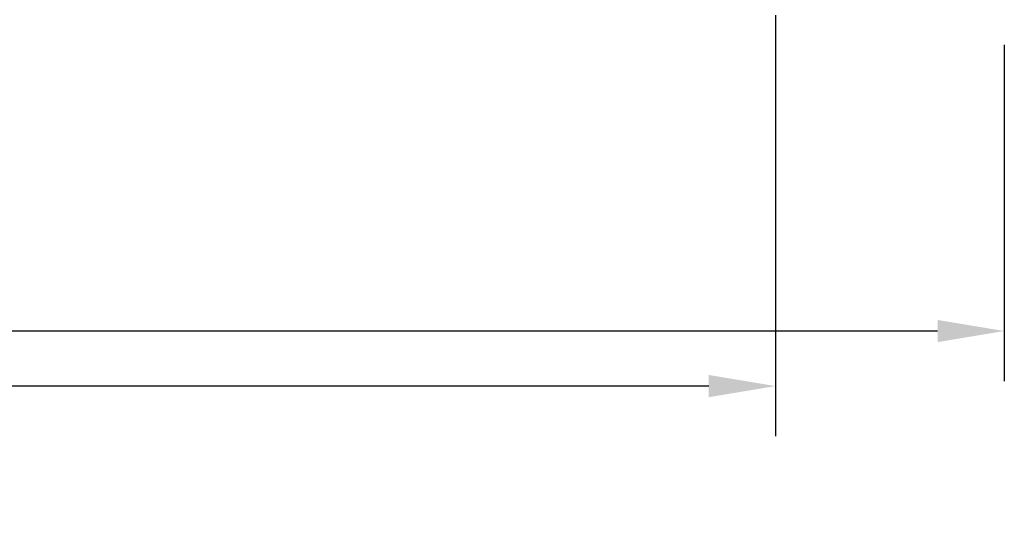
# Model space of a CAD drawing. Units: inches. Extents: x 89 to 490, y -59 to 378.
# Tile 13 of 20: x 400 to 459, y -59 to -28. Entities that reach past the tile are written whole.
import ezdxf

# ---------------------------------------------------------------- set-up
doc = ezdxf.new("R2010")
doc.units = ezdxf.units.IN
doc.header["$MEASUREMENT"] = 0
doc.layers.add('A-ANNO-DIMS', color=2, linetype='Continuous', lineweight=18)
doc.styles.get("Standard").update_dxf_attribs({"font": 'arial.ttf'})
doc.dimstyles.get("Standard").update_dxf_attribs({"dimtxt": 6, "dimasz": 4, "dimexe": 3, "dimexo": 3, "dimgap": 0.09, "dimtad": 0, "dimtih": 1, "dimtoh": 1, "dimdec": 1, "dimzin": 0, "dimdsep": 46, "dimlunit": 3, "dimtxsty": 'Standard', "dimcen": 0.09, "dimadec": 0, "dimazin": 0, "dimtfac": 1, "dimtdec": 1, "dimtofl": 0, "dimtmove": 0, "dimatfit": 3, "dimfxl": 1, "dimtolj": 1, "dimtzin": 0, "dimarcsym": 0})

# ---------------------------------------------------------------- blocks, each defined once
blk = doc.blocks.new('*D46')
at = {"layer": 'A-ANNO-DIMS', "color": 0, "lineweight": -2, "transparency": 16777216}
for p, q in [((277.443, -27.866), (277.443, -53.11)), ((445.739, -27.866), (445.739, -53.11)), ((281.443, -50.11), (332.892, -50.11)), ((441.739, -50.11), (390.289, -50.11))]:
    blk.add_line(p, q, dxfattribs=at)
at = {"layer": 'A-ANNO-DIMS', "color": 0, "transparency": 16777216}
for points in [[(281.443, -49.443), (281.443, -50.777), (277.443, -50.11)], [(441.739, -49.443), (441.739, -50.777), (445.739, -50.11)]]:
    blk.add_solid(points, dxfattribs=at)
at = {"layer": 'Defpoints', "color": 0, "transparency": 16777216}
for p in [(277.443, -24.866), (445.739, -24.866), (445.739, -50.11)]:
    blk.add_point(p, dxfattribs=at)
at = {"layer": 'A-ANNO-DIMS', "color": 0, "transparency": 16777216, "insert": (361.591, -50.11), "char_height": 6, "attachment_point": 5}
blk.add_mtext('\\A1;PLANTING 168', dxfattribs=at)
blk = doc.blocks.new('*D48')
at = {"layer": 'A-ANNO-DIMS', "color": 0, "lineweight": -2, "transparency": 16777216}
for p, q in [((127.441, 10.741), (127.441, -49.809)), ((459.441, -29.659), (459.441, -49.809)), ((131.441, -46.809), (286.756, -46.809)), ((455.441, -46.809), (300.127, -46.809))]:
    blk.add_line(p, q, dxfattribs=at)
at = {"layer": 'A-ANNO-DIMS', "color": 0, "transparency": 16777216}
for points in [[(131.441, -46.143), (131.441, -47.476), (127.441, -46.809)], [(455.441, -46.143), (455.441, -47.476), (459.441, -46.809)]]:
    blk.add_solid(points, dxfattribs=at)
at = {"layer": 'Defpoints', "color": 0, "transparency": 16777216}
for p in [(127.441, 13.741), (459.441, -26.659), (459.441, -46.809)]:
    blk.add_point(p, dxfattribs=at)
at = {"layer": 'A-ANNO-DIMS', "color": 0, "transparency": 16777216, "insert": (293.441, -46.809), "char_height": 6, "attachment_point": 5}
blk.add_mtext('\\A1;332', dxfattribs=at)

msp = doc.modelspace()

# ---------------------------------------------------------------- dimensions: what is measured, and where the dimension line sits
at = {"layer": 'A-ANNO-DIMS'}
dim = msp.add_linear_dim(base=(459.4414, -46.8094), p1=(127.4414, 13.7413), p2=(459.4414, -26.6594), dimstyle='Standard', override={"dimdec": 0, "dimlfac": 1, "dimrnd": 0, "dimzin": 0, "dimdsep": 46, "dimlunit": 2}, dxfattribs=at)
dim.commit()
dim.dimension.update_dxf_attribs({"geometry": '*D48', "text_midpoint": (293.4414, -46.8094)})
dim = msp.add_linear_dim(base=(445.7386, -50.11), p1=(277.443, -24.8656), p2=(445.7386, -24.8656), text='PLANTING <>', dimstyle='Standard', override={"dimdec": 0, "dimlfac": 1, "dimrnd": 0, "dimzin": 0, "dimdsep": 46, "dimlunit": 2}, dxfattribs=at)
dim.commit()
dim.dimension.update_dxf_attribs({"geometry": '*D46', "text_midpoint": (361.5908, -50.11)})

doc.saveas('drawing.dxf')
